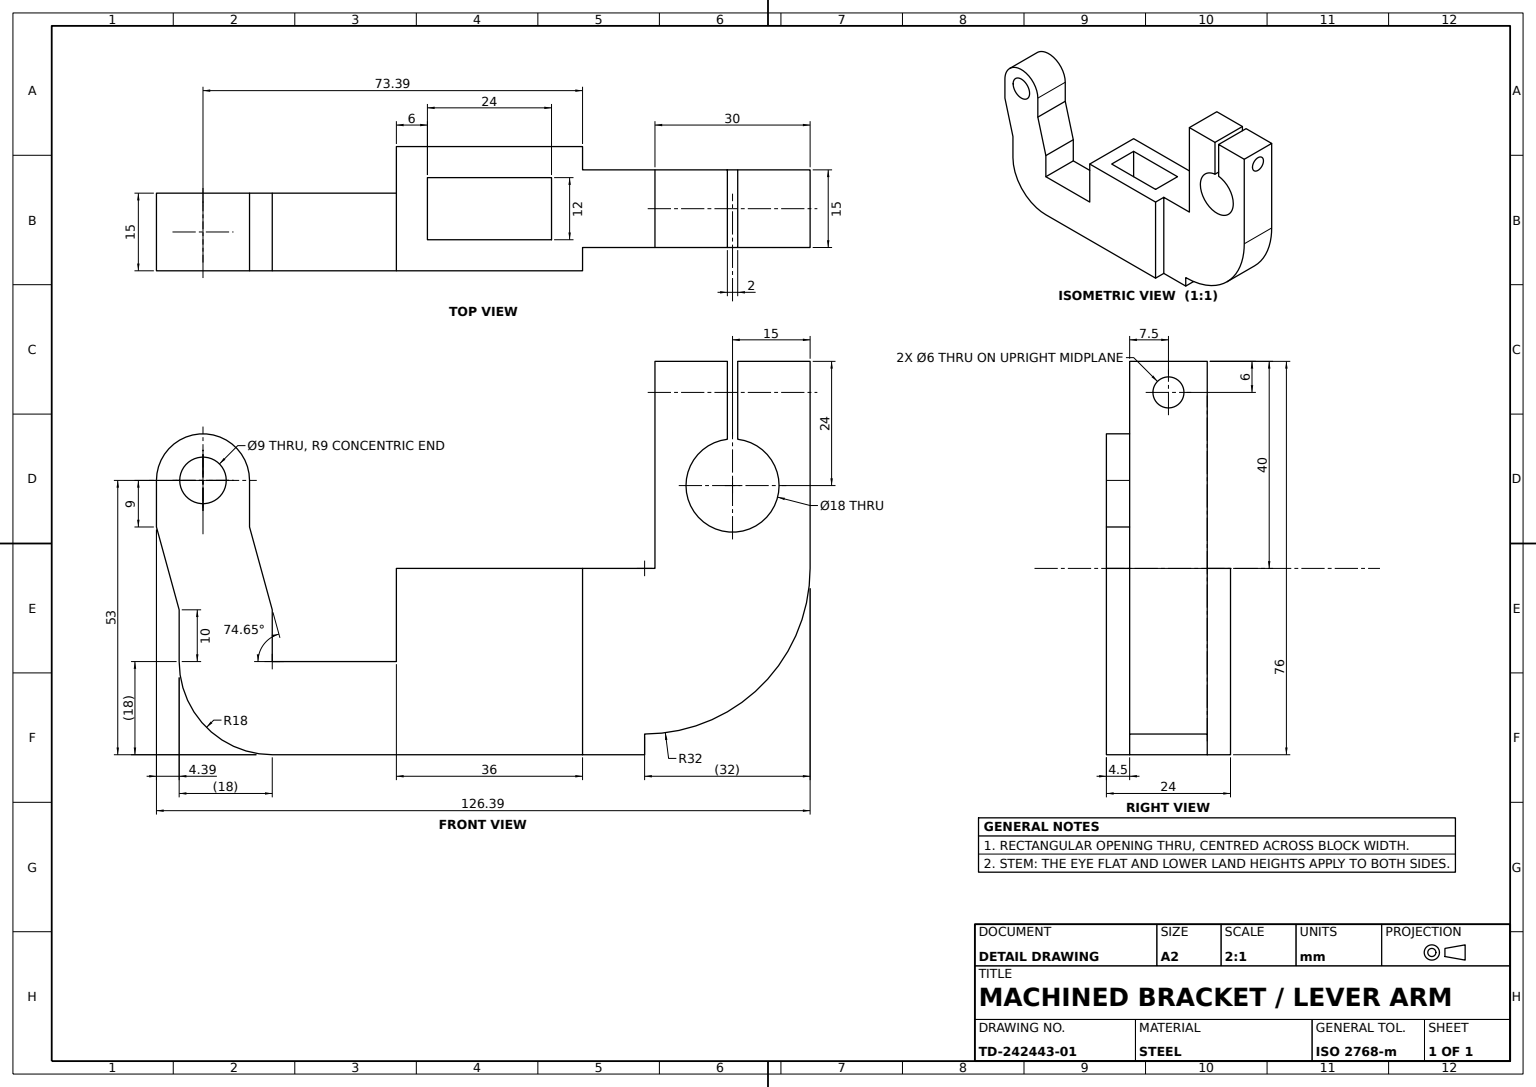
SolidWorks part; units mm, degrees
material "Plain Carbon Steel"
ref_plane "Front Plane" through (0, 0, 0) normal (0, 0, 1) x (1, 0, 0)
ref_plane "Top Plane" through (0, 0, 0) normal (0, 1, 0) x (1, 0, 0)
ref_plane "Right Plane" through (0, 0, 0) normal (1, 0, 0) x (0, 0, -1)
sketch "Base Block Sketch" plane through (0, 0, 0) normal (0, 1, 0) x (1, 0, 0)
  line L1 (-18, 12) -> (18, 12)
  line L2 (-18, 12) -> (-18, -12)
  line L3 (-18, -12) -> (18, -12)
  line L4 (18, 12) -> (18, -12)
  line L5 (-18, 12) -> (18, -12) construction
  line L6 (-18, -12) -> (18, 12) construction
  point P0 (0, 0)
  dimension "D1" = 36
  dimension "D2" = 24
extrude "Base Block" add sketch "Base Block Sketch" along normal blind 36
sketch "Rectangular Pocket Sketch" plane through (0, 36, 0) normal (0, 1, 0) x (1, 0, 0)
  line L1 (-12, 6) -> (12, 6)
  line L2 (-12, 6) -> (-12, -6)
  line L3 (-12, -6) -> (12, -6)
  line L4 (12, 6) -> (12, -6)
  line L5 (-12, 6) -> (12, -6) construction
  line L6 (-12, -6) -> (12, 6) construction
  point P0 (0, 0)
  dimension "D1" = 12
  dimension "D2" = 6
  dimension "D3" = 6
  dimension "D4" = 6
extrude "Rectangular Pocket 12x6" cut sketch "Rectangular Pocket Sketch" against normal through all both
sketch "Clamp Upright Sketch" plane through (0, 36, 0) normal (0, 1, 0) x (1, 0, 0)
  line L0 (-6.7112, 0) -> (37.5504, 0) construction
  line L1 (18, -12) -> (18, 12) construction
  line L2 (18, 7.5) -> (30, 7.5)
  line L3 (18, 7.5) -> (18, -7.5)
  line L4 (18, -7.5) -> (30, -7.5)
  line L5 (30, 7.5) -> (30, -7.5)
  dimension "D1" = 12
  dimension "D2" = 15
  dimension "D3" = 7.5
extrude "Clamp Upright" add sketch "Clamp Upright Sketch" against normal blind 36
sketch "Curved Arm Sketch" plane through (0, 0, 7.5) normal (0, 0, 1) x (1, 0, 0)
  line L1 (18, 36) -> (30, 36) construction
  line L2 (30, 0) -> (30, 36) construction
  line L4 (30, 36) -> (62, 36)
  line L5 (30, 4) -> (30, 36)
  arc A0 (30, 4) -> (62, 36) centre (30, 36) ccw
  dimension "D1" = 64
extrude "Curved Arm" add sketch "Curved Arm Sketch" against normal blind 15
sketch "Clamp Block Sketch" plane through (0, 36, 0) normal (0, 1, 0) x (1, 0, 0)
  line L0 (18, -7.5) -> (62, -7.5) construction
  line L1 (62, 7.5) -> (32, 7.5)
  line L2 (62, 7.5) -> (62, -7.5)
  line L3 (62, -7.5) -> (32, -7.5)
  line L4 (32, 7.5) -> (32, -7.5)
  dimension "D1" = 30
  dimension "D2" = 15
extrude "Clamp Block" add sketch "Clamp Block Sketch" along normal blind 40
sketch "Clamp Split Slot Sketch" plane through (0, 0, 7.5) normal (0, 0, 1) x (1, 0, 0)
  line L0 (23.2193, 52) -> (73.1254, 52) construction
  line L1 (32, 76) -> (62, 76) construction
  line L2 (47, 76) -> (47, 43.4913) construction
  line L3 (46, 76) -> (46, 60.9443)
  line L4 (48, 76) -> (48, 60.9443)
  line L5 (46, 76) -> (48, 76)
  line L8 (46, 76) -> (46, 43.4913) construction
  line L10 (48, 76) -> (48, 43.4913) construction
  arc A0 (46, 60.9443) -> (48, 60.9443) centre (47, 52) ccw
  dimension "D2" = 18
  dimension "D1" = 24
  dimension "D3" = 1
  dimension "D4" = 1
extrude "Clamp Split Slot 1mm" cut sketch "Clamp Split Slot Sketch" against normal through all both
sketch "Cross Hole Sketch" plane through (62, 0, 0) normal (1, 0, 0) x (0, 0, -1)
  line L0 (0, 76) -> (0, 70) construction
  line L1 (-7.5, 76) -> (7.5, 76) construction
  circle A0 centre (0, 70) radius 3
  dimension "D2" = 6
  dimension "D1" = 6
extrude "Clamp Cross Hole" cut sketch "Cross Hole Sketch" against normal through all both
sketch "Side Lug Sketch" plane through (0, 36, 0) normal (0, 1, 0) x (1, 0, 0)
  line L1 (-18, -12) -> (-42, -12)
  line L2 (-18, -12) -> (-18, 3)
  line L3 (-18, 3) -> (-42, 3)
  line L4 (-42, -12) -> (-42, 3)
  dimension "D1" = 15
  dimension "D2" = 24
extrude "Side Lug" add sketch "Side Lug Sketch" against normal blind 18 from offset 18 offset against normal yes
sketch "Arm Segment Sketch" plane through (0, 0, 12) normal (0, 0, 1) x (1, 0, 0)
  line L0 (-42, 18) -> (-42, 28)
  line L1 (-60, 18) -> (-60, 28)
  line L2 (-42, 0) -> (-42, 18) construction
  line L4 (-42, 0) -> (-42, 18)
  line L5 (-42, 28) -> (-60, 28)
  arc A0 (-60, 18) -> (-42, 0) centre (-42, 18) ccw
  dimension "D1" = 10
extrude "Arm Segment" add sketch "Arm Segment Sketch" against normal blind 15
sketch "Arm Link Sketch" plane through (0, 0, 12) normal (0, 0, 1) x (1, 0, 0)
  line L0 (-60, 28) -> (-42, 28)
  line L1 (-60, 28) -> (-64.3931, 44)
  line L2 (-42, 28) -> (-46.3931, 44)
  line L3 (-64.3931, 44) -> (-46.3931, 44)
  line L4 (18, 36) -> (18, 0) construction
  dimension "D1" = 16
  dimension "D2" = 64.3931
extrude "Arm Link" add sketch "Arm Link Sketch" against normal blind 15
sketch "Pivot Eye Sketch" plane through (0, 0, 12) normal (0, 0, 1) x (1, 0, 0)
  line L0 (-55.3931, 44) -> (-55.3931, 60.2634) construction
  line L2 (-64.3931, 44) -> (-64.3931, 53)
  line L3 (-64.3931, 44) -> (-46.3931, 44)
  line L4 (-46.3931, 53) -> (-46.3931, 44)
  line L5 (18, 36) -> (18, 0) construction
  line L6 (-42, 0) -> (18, 0) construction
  arc A0 (-46.3931, 53) -> (-64.3931, 53) centre (-55.3931, 53) ccw
  circle A1 centre (-55.3931, 53) radius 4.5
  dimension "D2" = 18
  dimension "D3" = 9
  dimension "D1" = 9
  dimension "D4" = 73.3931
  dimension "D5" = 44
extrude "Pivot Eye" add sketch "Pivot Eye Sketch" against normal blind 15
